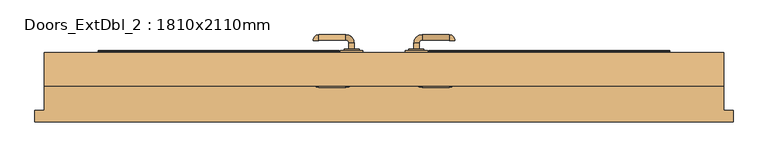
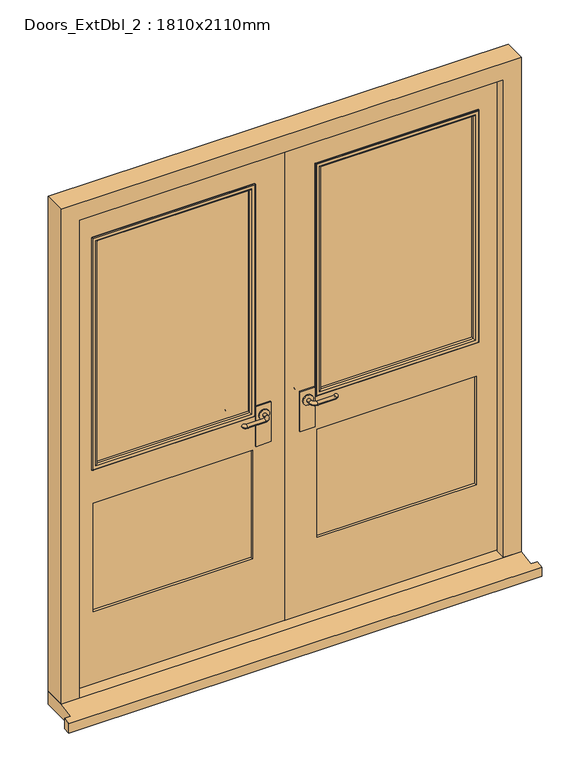
# IFC4 building model written with IfcOpenShell, lengths in millimetres: door geometry, Doors_ExtDbl_2 : 1810x2110mm.
# Revit data of these elements (continued)
# Type "Doors_ExtDbl_2 : 1810x2110mm" (continued)
#   Material Ironmongery = Door - Handle
#   Wall Closure = (empty or 0)
# Element 1 (IfcDoor, "Doors_ExtDbl_2 : 1810x2110mm")
#   Materials on its faces: "Door - Panel", "Door - Handle", "Door - Frame/Mullion", "Door - Glazing"
# Materials
#   "Door - Glazing": colour RGB 0 0 255, transparency 0.75
#   "Door - Panel": class "Wood", colour RGB 210 159 95, transparency 0, Cost = 0
#   "Door - Frame/Mullion": class "Wood", colour RGB 212 179 113, transparency 0
#   "Door - Handle": colour RGB 247 247 247, transparency 0
